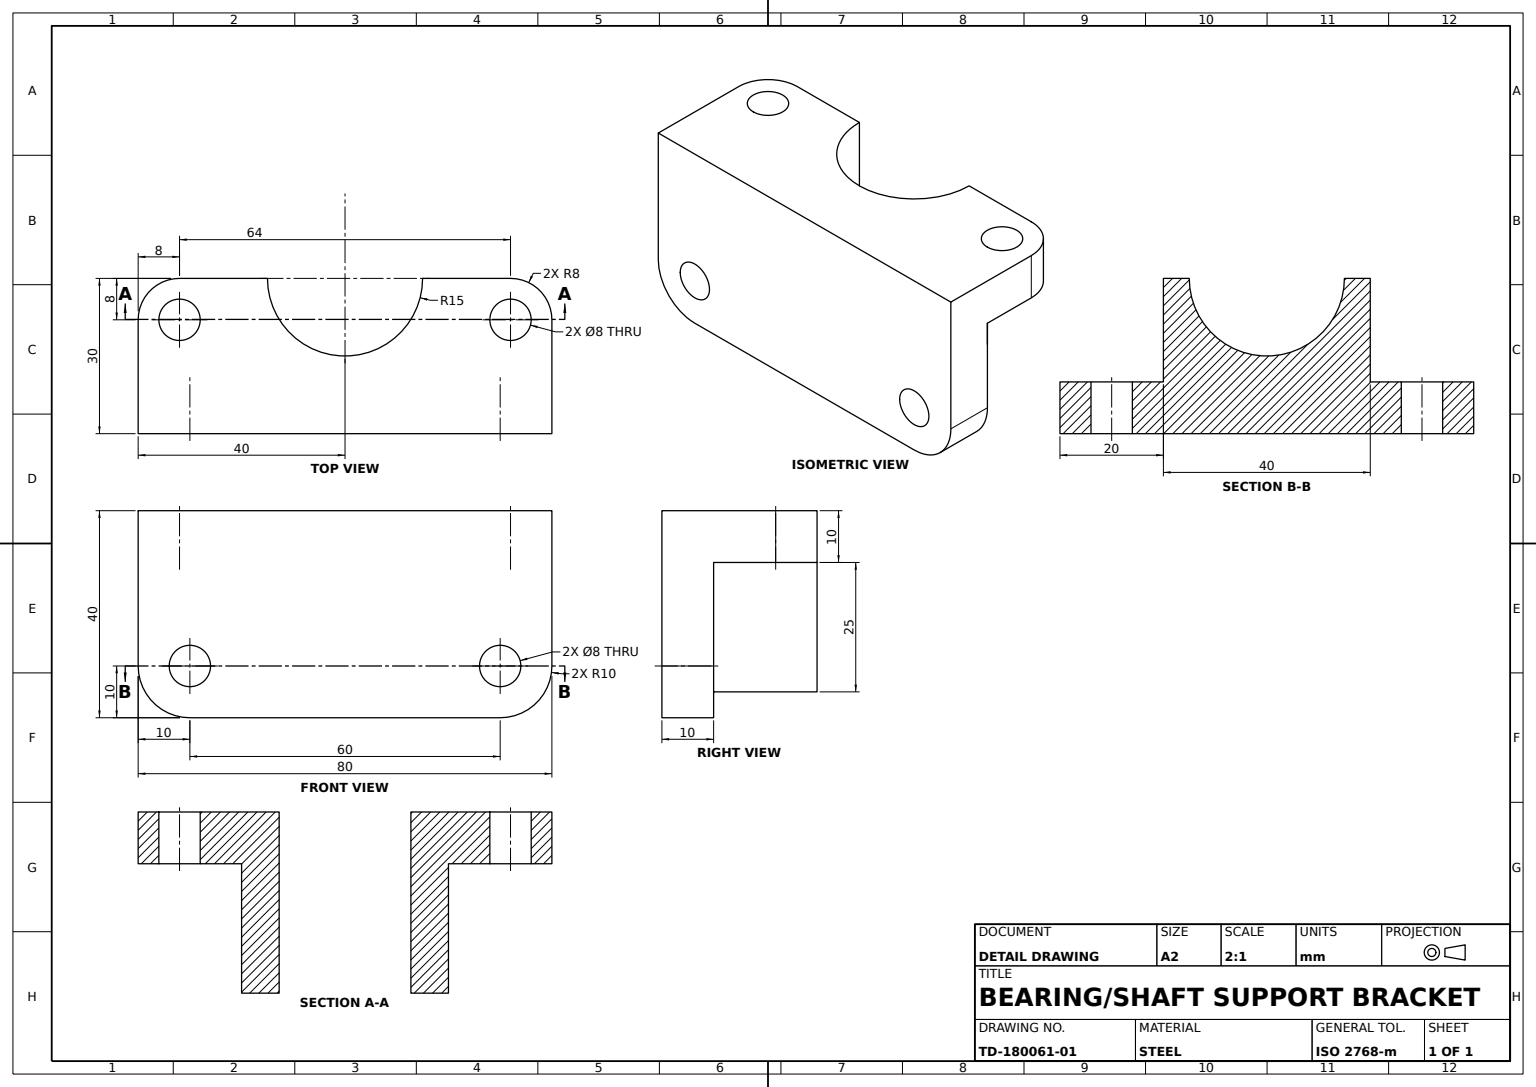
SolidWorks part; units mm, degrees
material "Plain Carbon Steel"
ref_plane "Front Plane" through (0, 0, 0) normal (0, 0, 1) x (1, 0, 0)
ref_plane "Top Plane" through (0, 0, 0) normal (0, 1, 0) x (1, 0, 0)
ref_plane "Right Plane" through (0, 0, 0) normal (1, 0, 0) x (0, 0, -1)
sketch "Base Plate Sketch" plane through (0, 0, 0) normal (0, 0, 1) x (1, 0, 0)
  line L0 (0, 0) -> (80, 0)
  line L1 (80, 0) -> (80, -30)
  line L2 (70, -40) -> (10, -40)
  line L3 (0, -30) -> (0, 0)
  arc A0 (70, -40) -> (80, -30) centre (70, -30) ccw
  arc A1 (10, -40) -> (0, -30) centre (10, -30) cw
  point P7 (80, -40)
  point P10 (0, -40)
  dimension "D4" = 10
  dimension "D1" = 80
  dimension "D2" = 40
  dimension "D3" = 80
extrude "Base Plate" add sketch "Base Plate Sketch" along normal blind 10
sketch "Lug Flange Sketch" plane through (0, 0, 0) normal (0, 1, 0) x (1, 0, 0)
  line L0 (8, 20) -> (72, 20)
  line L3 (80, 12) -> (80, 0)
  line L4 (80, 0) -> (0, 0)
  line L5 (0, 0) -> (0, 12)
  arc A0 (80, 12) -> (72, 20) centre (72, 12) ccw
  arc A1 (8, 20) -> (0, 12) centre (8, 12) ccw
  dimension "D1" = 8
  dimension "D2" = 20
extrude "Lug Flange" add sketch "Lug Flange Sketch" against normal blind 10
sketch "Saddle Block Sketch" plane through (0, -10, 0) normal (0, -1, 0) x (1, 0, 0)
  line L0 (40, 0) -> (60, 0)
  line L1 (0, 0) -> (80, 0) construction
  line L2 (20, 0) -> (20, -20)
  line L3 (40, 0) -> (20, 0)
  line L4 (72, -20) -> (8, -20) construction
  line L5 (20, -20) -> (60, -20)
  line L6 (60, -20) -> (60, 0)
  dimension "D1" = 20
  dimension "D2" = 40
  dimension "D3" = 20
extrude "Saddle Block" add sketch "Saddle Block Sketch" along normal blind 25
sketch "Cradle Sketch" plane through (0, -35, 0) normal (0, -1, 0) x (1, 0, 0)
  line L0 (20, -20) -> (60, -20) construction
  line L1 (25, -20) -> (55, -20)
  arc A0 (55, -20) -> (25, -20) centre (40, -20) ccw
  dimension "D1" = 30
extrude "Half-Round Cradle Cut" cut sketch "Cradle Sketch" against normal blind 35
sketch "Base Plate Lug Holes Sketch" plane through (0, 0, 0) normal (0, 0, -1) x (-1, 0, 0)
  circle A0 centre (-70, -30) radius 4
  circle A1 centre (-10, -30) radius 4
  dimension "D1" = 8
  dimension "D2" = 8
extrude "Base Plate Lug Holes 2x" cut sketch "Base Plate Lug Holes Sketch" against normal blind 35
sketch "Flange Lug Holes Sketch" plane through (0, -10, 0) normal (0, -1, 0) x (1, 0, 0)
  circle A0 centre (72, -12) radius 4
  circle A1 centre (8, -12) radius 4
  dimension "D1" = 8
  dimension "D2" = 8
extrude "Flange Lug Holes 2x" cut sketch "Flange Lug Holes Sketch" against normal blind 35
